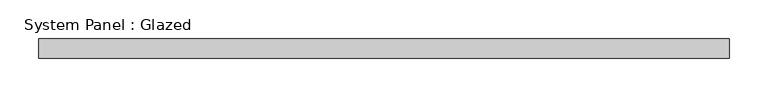
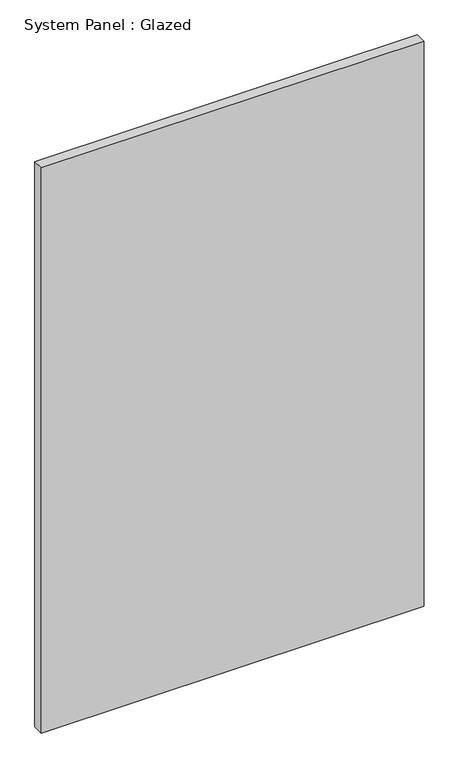
"""IFC4 building model written with IfcOpenShell, lengths in millimetres: plate geometry, System Panel : Glazed."""

from ifc_helpers import new_model, si_unit, origin, origin_with_axes, place, context, project, spatial, polyline, outline, extrude, source, transform, mapped, element, save


def system_panel_glazed_118543cb(model_context):
    return source(origin(), model_context, "Body", "SweptSolid", [
        extrude(outline(polyline([(447.675, 19.05), (-447.675, 19.05), (-447.675, 44.45), (447.675, 44.45), (447.675, 19.05)])), origin_with_axes(), (0.0, 0.0, 1.0), 1397.0),
    ])


if __name__ == "__main__":
    model = new_model("IFC4")
    model_context = context("Model", 3, world=origin())
    ifc_project = project(units=[si_unit("LENGTHUNIT", "METRE", prefix="MILLI")], contexts=[model_context])
    site = spatial("IfcSite", under=ifc_project)
    building = spatial("IfcBuilding", under=site)
    placement = place(None, origin())
    system_panel_glazed_shape = system_panel_glazed_118543cb(model_context)
    element("IfcPlate", 1, ObjectType="System Panel : Glazed", at=placement, inside=building, context=model_context, shape_type="MappedRepresentation", body=[
        mapped(system_panel_glazed_shape, transform((0.0, 0.0, 0.0), x_axis=(1.0, 0.0, 0.0), y_axis=(0.0, 1.0, 0.0), z_axis=(0.0, 0.0, 1.0))),
    ])
    save(model, "model.ifc")

# Revit data of these elements
# Type "System Panel : Glazed"
#   Construction Type Id = "GSP4R"
#   Analytic Construction = "1/8 in Pilkington single glazing"
#   Visual Light Transmittance = 0.9
#   Solar Heat Gain Coefficient = 0.86
#   Heat Transfer Coefficient (U) = 1.18115 BTU/(h·ft²·°F)
#   Define Thermal Properties by = 1
# Element 1 (IfcPlate, "System Panel : Glazed")
#   Materials on its faces: "Glass"
# Materials
#   "Glass": class "Glass", colour RGB 0 128 192, transparency 0.75, Description = "Soda Lime Glass", Cost = 0
